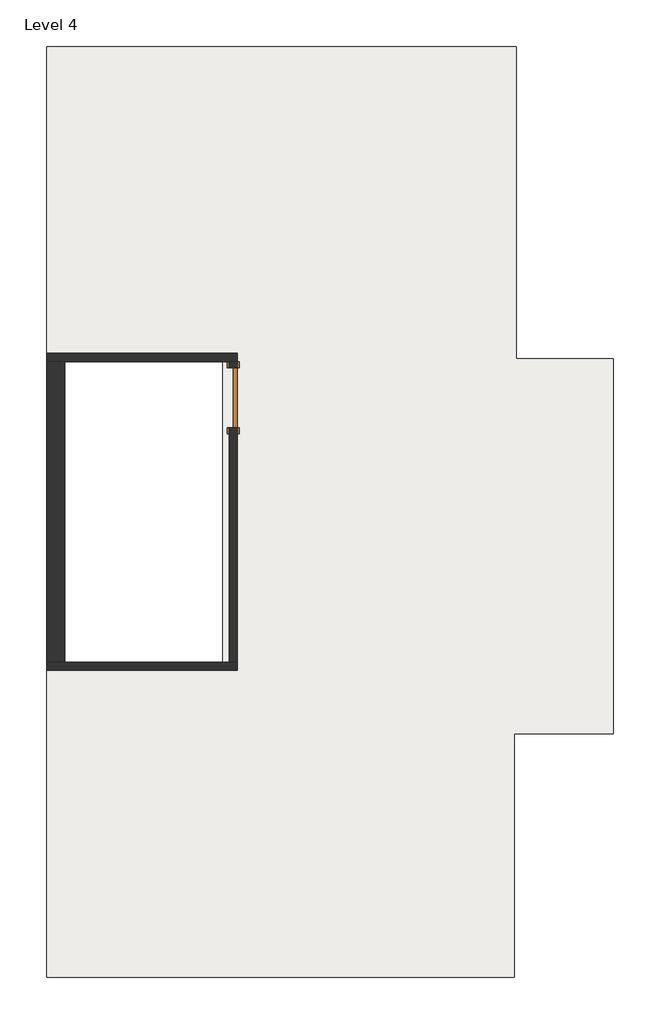
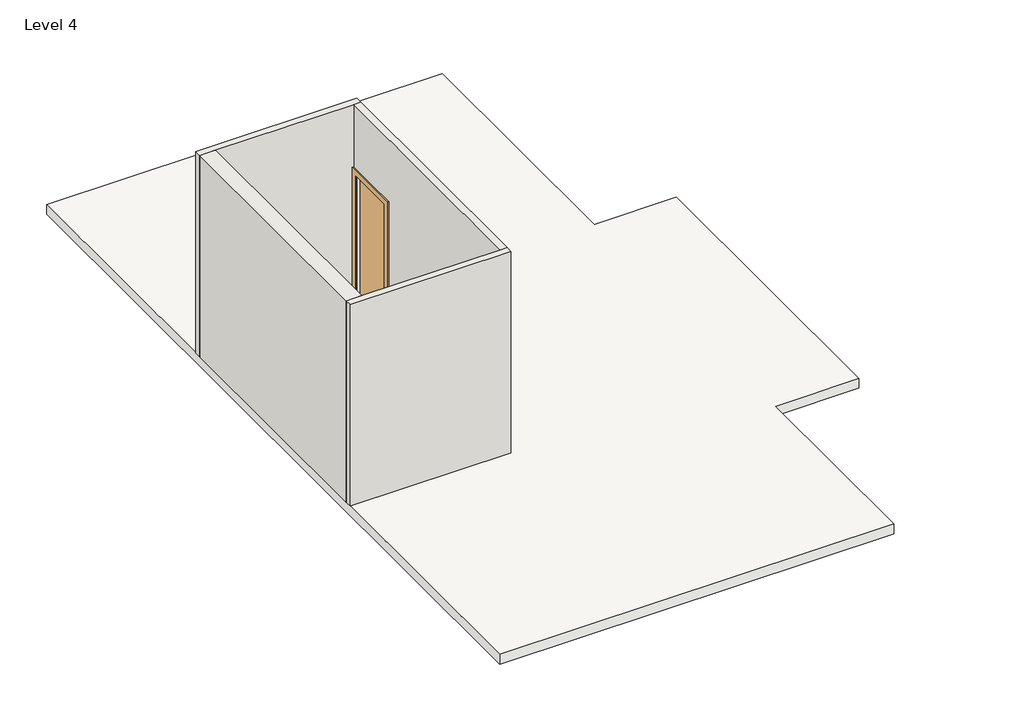
# One storey: 4 walls, 1 door, 1 slab.
"""IFC4 building model written with IfcOpenShell, lengths in millimetres."""

from ifc_helpers import new_model, si_unit, frame, origin, place, context, project, spatial, polyline, outline, extrude, faceted_brep, transform, mapped, element, save
from components import door_aa9e95e7

model = new_model("IFC4")

# Units and contexts
model_context = context("Model", 3, world=origin())
ifc_project = project(units=[si_unit("LENGTHUNIT", "METRE", prefix="MILLI")], contexts=[model_context])

# Site, building, storey
site = spatial("IfcSite", under=ifc_project)
building = spatial("IfcBuilding", under=site)
storey = spatial("IfcBuildingStorey", under=building, Name="Level 4", Elevation=7010.4)

# Door
placement = place(None, origin())
door_shape = door_aa9e95e7(model_context)
element("IfcDoor", 1, ObjectType="Single-Flush : 2'6\" x7'", at=placement, inside=storey, context=model_context, shape_type="MappedRepresentation", body=[
    mapped(door_shape, transform((-2700.1165653, 3152.9857557, 7010.4), x_axis=(0.0, 1.0, 0.0), y_axis=(-1.0, 0.0, 0.0), z_axis=(0.0, 0.0, 1.0))),
])

# Slab
element("IfcSlab", 2, ObjectType="6\" floor", at=placement, inside=storey, context=model_context, shape_type="SweptSolid", body=[
    extrude(outline(polyline([(-5062.3165653, 7597.9857557), (881.2834347, 7597.9857557), (881.2834347, 3648.2857557), (2113.1834347, 3648.2857557), (2113.1834347, -1101.5142443), (855.8834347, -1101.5142443), (855.8834347, -4187.6142443), (-5062.3165653, -4187.6142443), (-5062.3165653, 7597.9857557)]), holes=[polyline([(-2839.8165653, 3610.1857557), (-4833.7165653, 3610.1857557), (-4833.7165653, -199.8142443), (-2839.8165653, -199.8142443), (-2839.8165653, 3610.1857557)])]), frame((0.0, 0.0, 6858.0), z_axis=(0.0, 0.0, 1.0), x_axis=(1.0, 0.0, 0.0)), (0.0, 0.0, 1.0), 152.4),
])

# Walls
element("IfcWall", 3, at=placement, inside=storey, context=model_context, shape_type="Brep", body=[
    faceted_brep([(-5062.3165653, 3610.1857557, 7010.4), (-4833.7165653, 3610.1857557, 7010.4), (-2750.9165653, 3610.1857557, 7010.4), (-2649.3165653, 3610.1857557, 7010.4), (-2649.3165653, 3610.1857557, 10210.8), (-2750.9165653, 3610.1857557, 10210.8), (-4833.7165653, 3610.1857557, 10210.8), (-5062.3165653, 3610.1857557, 10210.8), (-5062.3165653, 3711.7857557, 7010.4), (-5062.3165653, 3711.7857557, 10210.8), (-2649.3165653, 3711.7857557, 10210.8), (-2649.3165653, 3711.7857557, 7010.4)], [[[0, 1, 2, 3, 4, 5, 6, 7]], [[8, 9, 10, 11]], [[3, 2, 1, 0, 8, 11]], [[7, 6, 5, 4, 10, 9]], [[4, 3, 11, 10]], [[0, 7, 9, 8]]]),
])
element("IfcWall", 4, at=placement, inside=storey, context=model_context, shape_type="Brep", body=[
    faceted_brep([(-5062.3165653, -301.4142443, 7010.4), (-2649.3165653, -301.4142443, 7010.4), (-2649.3165653, -301.4142443, 10210.8), (-5062.3165653, -301.4142443, 10210.8), (-5062.3165653, -199.8142443, 7010.4), (-5062.3165653, -199.8142443, 10210.8), (-4833.7165653, -199.8142443, 10210.8), (-2750.9165653, -199.8142443, 10210.8), (-2649.3165653, -199.8142443, 10210.8), (-2649.3165653, -199.8142443, 7010.4), (-2750.9165653, -199.8142443, 7010.4), (-4833.7165653, -199.8142443, 7010.4)], [[[0, 1, 2, 3]], [[4, 5, 6, 7, 8, 9, 10, 11]], [[1, 0, 4, 11, 10, 9]], [[3, 2, 8, 7, 6, 5]], [[2, 1, 9, 8]], [[0, 3, 5, 4]]]),
])
element("IfcWall", 5, at=placement, inside=storey, context=model_context, shape_type="SweptSolid", body=[
    extrude(outline(polyline([(3610.1857557, 7010.4), (3533.9857557, 7010.4), (3533.9857557, 9144.0), (2771.9857557, 9144.0), (2771.9857557, 7010.4), (-199.8142443, 7010.4), (-199.8142443, 10210.8), (3610.1857557, 10210.8), (3610.1857557, 7010.4)])), frame((-2750.9165653, 0.0, 0.0), z_axis=(1.0, 0.0, 0.0), x_axis=(0.0, 1.0, 0.0)), (0.0, 0.0, 1.0), 101.6),
])
element("IfcWall", 6, ObjectType="9\" wall", at=placement, inside=storey, context=model_context, shape_type="SweptSolid", body=[
    extrude(outline(polyline([(-5062.3165653, -199.8142443), (-5062.3165653, 3610.1857557), (-4833.7165653, 3610.1857557), (-4833.7165653, -199.8142443), (-5062.3165653, -199.8142443)])), frame((0.0, 0.0, 7010.4), z_axis=(0.0, 0.0, 1.0), x_axis=(1.0, 0.0, 0.0)), (0.0, 0.0, 1.0), 3200.4),
])

save(model, "model.ifc")

# Revit data of these elements
# Type "Single-Flush : 2'6\" x7'"
#   Type Mark = "15"
#   Construction Type Id = "MDOOR"
#   Assembly Code = "C1020"
#   Analytic Construction = "Metal"
#   Thickness = 0' - 2"
#   Heat Transfer Coefficient (U) = 0.651978 BTU/(h·ft²·°F)
#   Height = 7' - 0"
#   Trim Projection Ext = 0' - 1"
#   Trim Projection Int = 0' - 1"
#   Trim Width = 0' - 3"
#   Width = 2' - 6"
#   Define Thermal Properties by = 1
#   Door Material = Door - Panel
#   Frame Material = Door - Frame
#   Visual Light Transmittance = 0
#   Solar Heat Gain Coefficient = 0
#   Function = (empty or 0)
#   Wall Closure = (empty or 0)
# Type "6\" floor"
#   Assembly Code = "B1010"
#   Function = 0
#   Layers, outside or top first: 0' - 6" no material (function 1)
# Type
#   Assembly Code = "B2010"
#   Layers, outside or top first: 0' - 4" "01-9\" wall" (function 1)
# Type "9\" wall"
#   Assembly Code = "B2010"
#   Layers, outside or top first: 0' - 9" "01-9\" wall" (function 1)
# Element 1 (IfcDoor, "Single-Flush : 2'6\" x7'")
#   Phase Created = New Construction
#   Materials on its faces: "Door - Frame", "Door - Panel"
# Element 2 (IfcSlab, "6\" floor")
#   built-in parameter 1001955 = 3.14159 (stored number, unit not read)
#   Height Offset From Level = 0' - 0"
#   Phase Created = New Construction
#   Materials on its faces: "Default Floor"
# Elements 3, 4, 5 (IfcWall)
#   Top Offset = 0' - 0"
#   Base Offset = 0' - 0"
#   wall height = 10' - 6"
#   Phase Created = New Construction
#   Base Constraint = Level 4
#   Top Constraint = Level 5
#   Materials on its faces: "01-9\" wall"
# Element 6 (IfcWall, "9\" wall")
#   Top Offset = 0' - 0"
#   Base Offset = 0' - 0"
#   wall height = 10' - 6"
#   Phase Created = New Construction
#   Base Constraint = Level 4
#   Top Constraint = Level 5
#   Materials on its faces: "01-9\" wall"
# Materials
#   "Door - Panel": class "Wood", colour RGB 210 159 95, transparency 0, Cost = 0
#   "Door - Frame": colour RGB 118 70 51, transparency 0, Cost = 0
#   "01-9\" wall": class "Generic", colour RGB 244 244 244, transparency 0, Cost = 0
#   "Default Floor": colour RGB 128 128 128, transparency 0, Cost = 0
